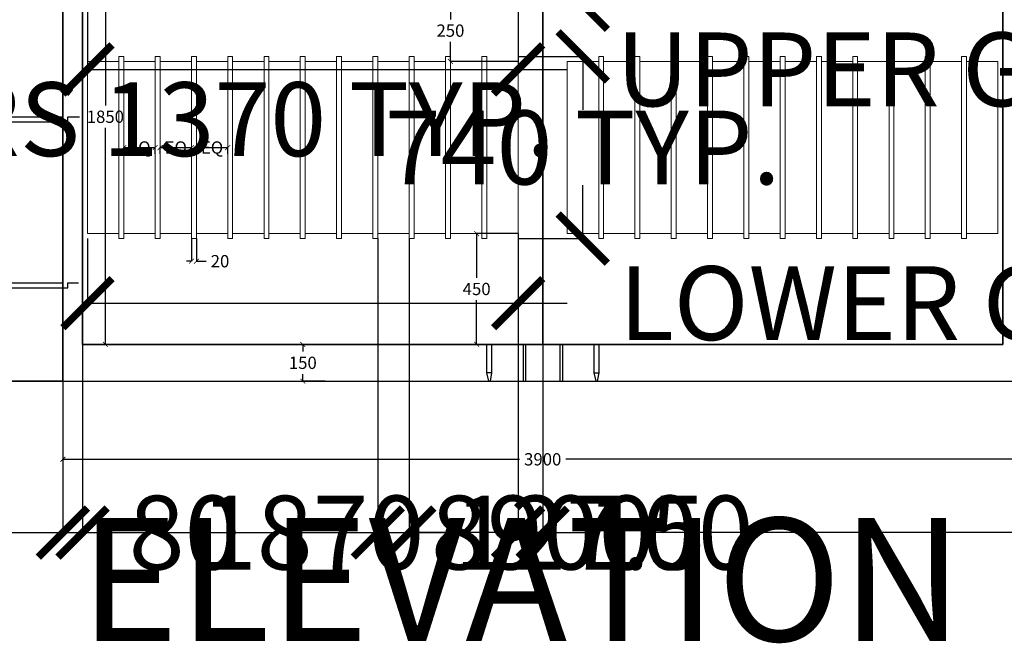
# Model space of a CAD drawing. Units: millimetres. Extents: x 16635 to 28332, y 17519 to 22633.
# Tile 2 of 4: x 20029 to 24031, y 17519 to 20054. Entities that reach past the tile are written whole.
import ezdxf
from ezdxf import colors
from ezdxf.entities.mleader import LeaderData, LeaderLine
from ezdxf.math import Vec2, Vec3

# ---------------------------------------------------------------- set-up
doc = ezdxf.new("R2010")
doc.units = ezdxf.units.MM
doc.header["$MEASUREMENT"] = 0
for name, color, linetype, lineweight in [('A-ANNO-DIMS', 2, 'Continuous', 18), ('A-ANNO-TEXT', 7, 'Continuous', 18), ('A-ELEV-GRAD', 7, 'Continuous', 30), ('A-GATE', 3, 'Continuous', 35), ('A-GATE-GRIL', 4, 'Continuous', 18), ('A-GATE-HRDW', 3, 'Continuous', 25), ('A-WALL', 7, 'Continuous', 35)]:
    doc.layers.add(name, color=color, linetype=linetype, lineweight=lineweight)
doc.styles.get("Standard").update_dxf_attribs({"font": 'arial.ttf'})
doc.dimstyles.get("Standard").update_dxf_attribs({"dimtxt": 300, "dimasz": 200, "dimexe": 0.18, "dimexo": 0.0625, "dimgap": 0.09, "dimtad": 0, "dimtih": 1, "dimtoh": 1, "dimdec": 0, "dimzin": 0, "dimdsep": 46, "dimtxsty": 'Standard', "dimblk": 'ARCHTICK', "dimcen": 0.09, "dimadec": 0, "dimazin": 0, "dimtfac": 1, "dimtdec": 0, "dimtofl": 0, "dimtmove": 0, "dimatfit": 3, "dimfxl": 1, "dimtolj": 1, "dimtzin": 0, "dimarcsym": 0})

# ---------------------------------------------------------------- blocks, each defined once
blk = doc.blocks.new('_ArchTick')
at = {"color": 0, "linetype": 'ByBlock', "const_width": 0.15}
blk.add_lwpolyline([(-0.5, -0.5), (0.5, 0.5)], dxfattribs=at)
blk = doc.blocks.new('*D13')
at = {"layer": 'A-ANNO-DIMS', "color": 0, "lineweight": -2, "transparency": 16777216}
for p, q in [((20284.8, 20584.3), (20377.6, 20584.3)), ((20377.4, 20584.3), (20377.4, 19704.9)), ((20377.4, 18734.3), (20377.4, 19613.8)), ((20284.8, 18734.3), (20377.6, 18734.3))]:
    blk.add_line(p, q, dxfattribs=at)
at = {"layer": 'Defpoints', "color": 0, "transparency": 16777216}
for p in [(20284.8, 20584.3), (20284.8, 18734.3), (20377.4, 18734.3)]:
    blk.add_point(p, dxfattribs=at)
at = {"layer": 'A-ANNO-DIMS', "color": 0, "lineweight": -2, "transparency": 16777216, "xscale": 20, "yscale": 20, "zscale": 20}
for p, rotation in [((20377.4, 20584.3), 90), ((20377.4, 18734.3), 270)]:
    blk.add_blockref('_ArchTick', p, dxfattribs=dict(at, rotation=rotation))
at = {"layer": 'A-ANNO-DIMS', "color": 0, "transparency": 16777216, "insert": (20377.4, 19659.3), "char_height": 50, "attachment_point": 5}
blk.add_mtext('\\A1;1850', dxfattribs=at)
blk = doc.blocks.new('*D14')
at = {"layer": 'A-ANNO-DIMS', "color": 0, "lineweight": -2, "transparency": 16777216}
for p, q in [((22054.7, 20134.3), (21779.6, 20134.3)), ((21779.8, 20134.3), (21779.8, 20054.9)), ((21779.8, 19884.3), (21779.8, 19963.8)), ((22054.7, 19884.3), (21779.6, 19884.3))]:
    blk.add_line(p, q, dxfattribs=at)
at = {"layer": 'Defpoints', "color": 0, "transparency": 16777216}
for p in [(22054.8, 20134.3), (21779.8, 19884.3), (22054.8, 19884.3)]:
    blk.add_point(p, dxfattribs=at)
at = {"layer": 'A-ANNO-DIMS', "color": 0, "lineweight": -2, "transparency": 16777216, "xscale": 20, "yscale": 20, "zscale": 20}
for p, rotation in [((21779.8, 20134.3), 90), ((21779.8, 19884.3), 270)]:
    blk.add_blockref('_ArchTick', p, dxfattribs=dict(at, rotation=rotation))
at = {"layer": 'A-ANNO-DIMS', "color": 0, "transparency": 16777216, "insert": (21779.8, 20009.3), "char_height": 50, "attachment_point": 5}
blk.add_mtext('\\A1;250', dxfattribs=at)
blk = doc.blocks.new('*D16')
at = {"layer": 'A-ANNO-DIMS', "color": 0, "lineweight": -2, "transparency": 16777216}
for p, q in [((21271.2, 18734.3), (21179.6, 18734.3)), ((21179.8, 18734.3), (21179.8, 18704.9)), ((21179.8, 18584.3), (21179.8, 18613.8)), ((21271.2, 18584.3), (21179.6, 18584.3))]:
    blk.add_line(p, q, dxfattribs=at)
at = {"layer": 'Defpoints', "color": 0, "transparency": 16777216}
for p in [(21179.8, 18734.3), (21271.2, 18734.3), (21271.2, 18584.3)]:
    blk.add_point(p, dxfattribs=at)
at = {"layer": 'A-ANNO-DIMS', "color": 0, "lineweight": -2, "transparency": 16777216, "xscale": 20, "yscale": 20, "zscale": 20}
for p, rotation in [((21179.8, 18734.3), 90), ((21179.8, 18584.3), 270)]:
    blk.add_blockref('_ArchTick', p, dxfattribs=dict(at, rotation=rotation))
at = {"layer": 'A-ANNO-DIMS', "color": 0, "transparency": 16777216, "insert": (21179.8, 18659.3), "char_height": 50, "attachment_point": 5}
blk.add_mtext('\\A1;150', dxfattribs=at)
blk = doc.blocks.new('*D17')
at = {"layer": 'A-ANNO-DIMS', "color": 0, "lineweight": -2, "transparency": 16777216}
for p, q in [((22054.7, 19184.3), (21886.1, 19184.3)), ((21886.3, 19184.3), (21886.3, 19004.9)), ((21886.3, 18734.3), (21886.3, 18913.8)), ((22054.7, 18734.3), (21886.1, 18734.3))]:
    blk.add_line(p, q, dxfattribs=at)
at = {"layer": 'Defpoints', "color": 0, "transparency": 16777216}
for p in [(22054.8, 19184.3), (21886.3, 18734.3), (22054.8, 18734.3)]:
    blk.add_point(p, dxfattribs=at)
at = {"layer": 'A-ANNO-DIMS', "color": 0, "lineweight": -2, "transparency": 16777216, "xscale": 20, "yscale": 20, "zscale": 20}
for p, rotation in [((21886.3, 19184.3), 90), ((21886.3, 18734.3), 270)]:
    blk.add_blockref('_ArchTick', p, dxfattribs=dict(at, rotation=rotation))
at = {"layer": 'A-ANNO-DIMS', "color": 0, "transparency": 16777216, "insert": (21886.3, 18959.3), "char_height": 50, "attachment_point": 5}
blk.add_mtext('\\A1;450', dxfattribs=at)
blk = doc.blocks.new('*D19')
at = {"layer": 'A-ANNO-DIMS', "color": 0, "lineweight": -2, "transparency": 16777216}
for p, q in [((20204.8, 18584.3), (20204.8, 18267)), ((24104.8, 18584.3), (24104.8, 18267)), ((20204.8, 18267.2), (22060.2, 18267.2)), ((24104.8, 18267.2), (22249.3, 18267.2))]:
    blk.add_line(p, q, dxfattribs=at)
at = {"layer": 'Defpoints', "color": 0, "transparency": 16777216}
for p in [(20204.8, 18584.3), (24104.8, 18584.3), (24104.8, 18267.2)]:
    blk.add_point(p, dxfattribs=at)
at = {"layer": 'A-ANNO-DIMS', "color": 0, "lineweight": -2, "transparency": 16777216, "xscale": 20, "yscale": 20, "zscale": 20, "rotation": 180}
blk.add_blockref('_ArchTick', (20204.8, 18267.2), dxfattribs=at)
at = {"layer": 'A-ANNO-DIMS', "color": 0, "lineweight": -2, "transparency": 16777216, "xscale": 20, "yscale": 20, "zscale": 20}
blk.add_blockref('_ArchTick', (24104.8, 18267.2), dxfattribs=at)
at = {"layer": 'A-ANNO-DIMS', "color": 0, "transparency": 16777216, "insert": (22154.8, 18267.2), "char_height": 50, "attachment_point": 5}
blk.add_mtext('\\A1;3900', dxfattribs=at)
blk = doc.blocks.new('*D28')
at = {"layer": 'A-ANNO-DIMS', "color": 0, "lineweight": -2, "transparency": 16777216}
for p, q in [((20727.3, 19164.3), (20727.3, 19072.1)), ((20747.3, 19164.3), (20747.3, 19072.1)), ((20727.3, 19072.3), (20707.3, 19072.3)), ((20747.3, 19072.3), (20787.3, 19072.3))]:
    blk.add_line(p, q, dxfattribs=at)
at = {"layer": 'Defpoints', "color": 0, "transparency": 16777216}
for p in [(20727.3, 19164.3), (20747.3, 19164.3), (20747.3, 19072.3)]:
    blk.add_point(p, dxfattribs=at)
at = {"layer": 'A-ANNO-DIMS', "color": 0, "lineweight": -2, "transparency": 16777216, "xscale": 20, "yscale": 20, "zscale": 20}
blk.add_blockref('_ArchTick', (20727.3, 19072.3), dxfattribs=at)
at = {"layer": 'A-ANNO-DIMS', "color": 0, "lineweight": -2, "transparency": 16777216, "xscale": 20, "yscale": 20, "zscale": 20, "rotation": 180}
blk.add_blockref('_ArchTick', (20747.3, 19072.3), dxfattribs=at)
at = {"layer": 'A-ANNO-DIMS', "color": 0, "transparency": 16777216, "insert": (20843.4, 19072.3), "char_height": 50, "attachment_point": 5}
blk.add_mtext('\\A1;20', dxfattribs=at)
blk = doc.blocks.new('*D32')
at = {"layer": 'A-ANNO-DIMS', "color": 0, "lineweight": -2, "transparency": 16777216}
for p, q in [((20452.3, 19508.7), (20452.3, 19534.5)), ((20452.3, 19534.3), (20579.8, 19534.3)), ((20579.8, 19508.7), (20579.8, 19534.5))]:
    blk.add_line(p, q, dxfattribs=at)
at = {"layer": 'Defpoints', "color": 0, "transparency": 16777216}
for p in [(20579.8, 19534.3), (20452.3, 19508.6), (20579.8, 19508.6)]:
    blk.add_point(p, dxfattribs=at)
at = {"layer": 'A-ANNO-DIMS', "color": 0, "lineweight": -2, "transparency": 16777216, "xscale": 20, "yscale": 20, "zscale": 20, "rotation": 180}
blk.add_blockref('_ArchTick', (20452.3, 19534.3), dxfattribs=at)
at = {"layer": 'A-ANNO-DIMS', "color": 0, "lineweight": -2, "transparency": 16777216, "xscale": 20, "yscale": 20, "zscale": 20}
blk.add_blockref('_ArchTick', (20579.8, 19534.3), dxfattribs=at)
at = {"layer": 'A-ANNO-DIMS', "color": 0, "transparency": 16777216, "insert": (20516, 19534.3), "char_height": 50, "attachment_point": 5}
blk.add_mtext('\\A1;EQ', dxfattribs=at)
blk = doc.blocks.new('*D33')
at = {"layer": 'A-ANNO-DIMS', "color": 0, "lineweight": -2, "transparency": 16777216}
for p, q in [((20599.8, 19508.7), (20599.8, 19534.5)), ((20599.8, 19534.3), (20727.3, 19534.3)), ((20727.3, 19508.7), (20727.3, 19534.5))]:
    blk.add_line(p, q, dxfattribs=at)
at = {"layer": 'Defpoints', "color": 0, "transparency": 16777216}
for p in [(20727.3, 19534.3), (20599.8, 19508.6), (20727.3, 19508.6)]:
    blk.add_point(p, dxfattribs=at)
at = {"layer": 'A-ANNO-DIMS', "color": 0, "lineweight": -2, "transparency": 16777216, "xscale": 20, "yscale": 20, "zscale": 20, "rotation": 180}
blk.add_blockref('_ArchTick', (20599.8, 19534.3), dxfattribs=at)
at = {"layer": 'A-ANNO-DIMS', "color": 0, "lineweight": -2, "transparency": 16777216, "xscale": 20, "yscale": 20, "zscale": 20}
blk.add_blockref('_ArchTick', (20727.3, 19534.3), dxfattribs=at)
at = {"layer": 'A-ANNO-DIMS', "color": 0, "transparency": 16777216, "insert": (20663.5, 19534.3), "char_height": 50, "attachment_point": 5}
blk.add_mtext('\\A1;EQ', dxfattribs=at)
blk = doc.blocks.new('*D34')
at = {"layer": 'A-ANNO-DIMS', "color": 0, "lineweight": -2, "transparency": 16777216}
for p, q in [((20747.3, 19508.7), (20747.3, 19534.5)), ((20747.3, 19534.3), (20874.8, 19534.3)), ((20874.8, 19508.7), (20874.8, 19534.5))]:
    blk.add_line(p, q, dxfattribs=at)
at = {"layer": 'Defpoints', "color": 0, "transparency": 16777216}
for p in [(20874.8, 19534.3), (20747.3, 19508.6), (20874.8, 19508.6)]:
    blk.add_point(p, dxfattribs=at)
at = {"layer": 'A-ANNO-DIMS', "color": 0, "lineweight": -2, "transparency": 16777216, "xscale": 20, "yscale": 20, "zscale": 20, "rotation": 180}
blk.add_blockref('_ArchTick', (20747.3, 19534.3), dxfattribs=at)
at = {"layer": 'A-ANNO-DIMS', "color": 0, "lineweight": -2, "transparency": 16777216, "xscale": 20, "yscale": 20, "zscale": 20}
blk.add_blockref('_ArchTick', (20874.8, 19534.3), dxfattribs=at)
at = {"layer": 'A-ANNO-DIMS', "color": 0, "transparency": 16777216, "insert": (20811, 19534.3), "char_height": 50, "attachment_point": 5}
blk.add_mtext('\\A1;EQ', dxfattribs=at)
blk = doc.blocks.new('GATE-GRILLE-LOWER')
for p, q in [((127.5, 720), (127.5, 740)), ((127.5, 740), (147.5, 740)), ((147.5, 740), (147.5, 720)), ((275, 720), (275, 740)), ((275, 740), (295, 740)), ((295, 740), (295, 720)), ((422.5, 720), (422.5, 740)), ((422.5, 740), (442.5, 740)), ((442.5, 740), (442.5, 720)), ((570, 720), (570, 740)), ((570, 740), (590, 740)), ((590, 740), (590, 720)), ((717.5, 720), (717.5, 740)), ((717.5, 740), (737.5, 740)), ((737.5, 740), (737.5, 720)), ((865, 720), (865, 740)), ((865, 740), (885, 740)), ((885, 740), (885, 720)), ((1012.5, 720), (1012.5, 740)), ((1012.5, 740), (1032.5, 740)), ((1032.5, 740), (1032.5, 720)), ((1160, 720), (1160, 740)), ((1160, 740), (1180, 740)), ((1180, 740), (1180, 720)), ((1307.5, 720), (1307.5, 740)), ((1307.5, 740), (1327.5, 740)), ((1327.5, 740), (1327.5, 720)), ((1455, 720), (1455, 740)), ((1455, 740), (1475, 740)), ((1475, 740), (1475, 720)), ((1602.5, 720), (1602.5, 740)), ((1602.5, 740), (1622.5, 740)), ((1622.5, 740), (1622.5, 720)), ((0, 720), (127.5, 720)), ((0, 720), (0, 20)), ((127.5, 720), (127.5, 20)), ((147.5, 720), (147.5, 20)), ((147.5, 720), (275, 720)), ((275, 720), (275, 20)), ((295, 720), (295, 20)), ((295, 720), (422.5, 720)), ((422.5, 720), (422.5, 20)), ((442.5, 720), (442.5, 20)), ((442.5, 720), (570, 720)), ((570, 720), (570, 20)), ((590, 720), (590, 20)), ((590, 720), (717.5, 720)), ((717.5, 720), (717.5, 20)), ((737.5, 720), (737.5, 20)), ((737.5, 720), (865, 720)), ((865, 720), (865, 20)), ((885, 720), (885, 20)), ((885, 720), (1012.5, 720)), ((1012.5, 720), (1012.5, 20)), ((1032.5, 720), (1032.5, 20)), ((1032.5, 720), (1160, 720)), ((1160, 720), (1160, 20)), ((1180, 720), (1180, 20)), ((1180, 720), (1307.5, 720)), ((1307.5, 720), (1307.5, 20)), ((1327.5, 720), (1327.5, 20)), ((1327.5, 720), (1455, 720)), ((1455, 720), (1455, 20)), ((1475, 720), (1475, 20)), ((1475, 720), (1602.5, 720)), ((1602.5, 720), (1602.5, 20)), ((1622.5, 720), (1622.5, 20)), ((1622.5, 720), (1750, 720)), ((1750, 720), (1750, 20)), ((0, 20), (127.5, 20)), ((127.5, 20), (127.5, 0)), ((147.5, 0), (147.5, 20)), ((147.5, 20), (275, 20)), ((275, 20), (275, 0)), ((295, 0), (295, 20)), ((295, 20), (422.5, 20)), ((422.5, 20), (422.5, 0)), ((442.5, 0), (442.5, 20)), ((442.5, 20), (570, 20)), ((570, 20), (570, 0)), ((590, 0), (590, 20)), ((590, 20), (717.5, 20)), ((717.5, 20), (717.5, 0)), ((737.5, 0), (737.5, 20)), ((737.5, 20), (865, 20)), ((865, 20), (865, 0)), ((885, 0), (885, 20)), ((885, 20), (1012.5, 20)), ((1012.5, 20), (1012.5, 0)), ((1032.5, 0), (1032.5, 20)), ((1032.5, 20), (1160, 20)), ((1160, 20), (1160, 0)), ((1180, 0), (1180, 20)), ((1180, 20), (1307.5, 20)), ((1307.5, 20), (1307.5, 0)), ((1327.5, 0), (1327.5, 20)), ((1327.5, 20), (1455, 20)), ((1455, 20), (1455, 0)), ((1475, 0), (1475, 20)), ((1475, 20), (1602.5, 20)), ((1602.5, 20), (1602.5, 0)), ((1622.5, 0), (1622.5, 20)), ((1622.5, 20), (1750, 20)), ((127.5, 0), (147.5, 0)), ((275, 0), (295, 0)), ((422.5, 0), (442.5, 0)), ((570, 0), (590, 0)), ((717.5, 0), (737.5, 0)), ((865, 0), (885, 0)), ((1012.5, 0), (1032.5, 0)), ((1160, 0), (1180, 0)), ((1307.5, 0), (1327.5, 0)), ((1455, 0), (1475, 0)), ((1602.5, 0), (1622.5, 0))]:
    blk.add_line(p, q)
blk = doc.blocks.new('GATE-JAMB-ANCHOR-SET')
for p, q in [((0.2, 1370), (297.2, 1370)), ((317.2, 1350), (317.2, 1370)), ((317.2, 1370), (351.9, 1370)), ((0.2, 1350), (297.2, 1350)), ((297.2, 1350), (317.2, 1350)), ((0, 694.8), (297, 694.8)), ((317, 674.8), (317, 694.8)), ((317, 694.8), (365.3, 694.8)), ((0, 674.8), (297, 674.8)), ((297, 674.8), (317, 674.8)), ((0.2, 20), (297.2, 20)), ((317.2, 0), (317.2, 20)), ((317.2, 20), (360.9, 20)), ((0.2, 0), (297.2, 0)), ((297.2, 0), (317.2, 0))]:
    blk.add_line(p, q)
blk = doc.blocks.new('*D43')
at = {"layer": 'A-ANNO-DIMS', "color": 0, "lineweight": -2, "transparency": 16777216}
for p, q in [((20304.8, 19164.3), (20304.8, 18901.7)), ((22054.8, 19164.3), (22054.8, 18901.7)), ((20304.8, 18901.8), (22054.8, 18901.8)), ((22054.8, 18901.8), (22254.8, 18901.8))]:
    blk.add_line(p, q, dxfattribs=at)
at = {"layer": 'Defpoints', "color": 0, "transparency": 16777216}
for p in [(20304.8, 19164.3), (22054.8, 19164.3), (22054.8, 18901.8)]:
    blk.add_point(p, dxfattribs=at)
at = {"layer": 'A-ANNO-DIMS', "color": 0, "lineweight": -2, "transparency": 16777216, "xscale": 200, "yscale": 200, "zscale": 200, "rotation": 180}
blk.add_blockref('_ArchTick', (20304.8, 18901.8), dxfattribs=at)
at = {"layer": 'A-ANNO-DIMS', "color": 0, "lineweight": -2, "transparency": 16777216, "xscale": 200, "yscale": 200, "zscale": 200}
blk.add_blockref('_ArchTick', (22054.8, 18901.8), dxfattribs=at)
at = {"layer": 'A-ANNO-DIMS', "color": 0, "transparency": 16777216, "insert": (24841.7, 18901.8), "char_height": 300, "attachment_point": 5}
blk.add_mtext('\\A1;LOWER GRILLE 1750 TYP.', dxfattribs=at)
blk = doc.blocks.new('*D44')
at = {"layer": 'A-ANNO-DIMS', "color": 0, "lineweight": -2, "transparency": 16777216}
for p, q in [((22054.8, 19904.3), (22317.5, 19904.3)), ((22317.3, 19904.3), (22317.3, 19687.6)), ((22317.3, 19164.3), (22317.3, 19381.1)), ((22054.8, 19164.3), (22317.5, 19164.3))]:
    blk.add_line(p, q, dxfattribs=at)
at = {"layer": 'Defpoints', "color": 0, "transparency": 16777216}
for p in [(22054.8, 19904.3), (22317.3, 19904.3), (22054.8, 19164.3)]:
    blk.add_point(p, dxfattribs=at)
at = {"layer": 'A-ANNO-DIMS', "color": 0, "lineweight": -2, "transparency": 16777216, "xscale": 200, "yscale": 200, "zscale": 200}
for p, rotation in [((22317.3, 19904.3), 90), ((22317.3, 19164.3), 270)]:
    blk.add_blockref('_ArchTick', p, dxfattribs=dict(at, rotation=rotation))
at = {"layer": 'A-ANNO-DIMS', "color": 0, "transparency": 16777216, "insert": (22317.3, 19534.3), "char_height": 300, "attachment_point": 5}
blk.add_mtext('\\A1;740 TYP.', dxfattribs=at)
blk = doc.blocks.new('*D45')
at = {"layer": 'A-ANNO-DIMS', "color": 0, "lineweight": -2, "transparency": 16777216}
for p, q in [((20304.8, 20114.3), (20304.8, 19851.7)), ((22054.8, 20114.3), (22054.8, 19851.7)), ((20304.8, 19851.8), (22054.8, 19851.8)), ((22054.8, 19851.8), (22254.8, 19851.8))]:
    blk.add_line(p, q, dxfattribs=at)
at = {"layer": 'Defpoints', "color": 0, "transparency": 16777216}
for p in [(20304.8, 20114.3), (22054.8, 20114.3), (22054.8, 19851.8)]:
    blk.add_point(p, dxfattribs=at)
at = {"layer": 'A-ANNO-DIMS', "color": 0, "lineweight": -2, "transparency": 16777216, "xscale": 200, "yscale": 200, "zscale": 200, "rotation": 180}
blk.add_blockref('_ArchTick', (20304.8, 19851.8), dxfattribs=at)
at = {"layer": 'A-ANNO-DIMS', "color": 0, "lineweight": -2, "transparency": 16777216, "xscale": 200, "yscale": 200, "zscale": 200}
blk.add_blockref('_ArchTick', (22054.8, 19851.8), dxfattribs=at)
at = {"layer": 'A-ANNO-DIMS', "color": 0, "transparency": 16777216, "insert": (24794.1, 19851.8), "char_height": 300, "attachment_point": 5}
blk.add_mtext('\\A1;UPPER GRILLE 1750 TYP.', dxfattribs=at)
blk = doc.blocks.new('*D46')
at = {"layer": 'A-ANNO-DIMS', "color": 0, "lineweight": -2, "transparency": 16777216}
for p, q in [((22054.8, 20525.3), (22317.5, 20525.3)), ((22317.3, 20525.3), (22317.3, 20470.7)), ((22317.3, 20114.3), (22317.3, 20169)), ((22054.8, 20114.3), (22317.5, 20114.3))]:
    blk.add_line(p, q, dxfattribs=at)
at = {"layer": 'Defpoints', "color": 0, "transparency": 16777216}
for p in [(22054.8, 20525.3), (22317.3, 20525.3), (22054.8, 20114.3)]:
    blk.add_point(p, dxfattribs=at)
at = {"layer": 'A-ANNO-DIMS', "color": 0, "lineweight": -2, "transparency": 16777216, "xscale": 200, "yscale": 200, "zscale": 200}
for p, rotation in [((22317.3, 20525.3), 90), ((22317.3, 20114.3), 270)]:
    blk.add_blockref('_ArchTick', p, dxfattribs=dict(at, rotation=rotation))
at = {"layer": 'A-ANNO-DIMS', "color": 0, "transparency": 16777216, "insert": (22317.3, 20319.8), "char_height": 300, "attachment_point": 5}
blk.add_mtext('\\A1;411 TYP.', dxfattribs=at)
blk = doc.blocks.new('*D47')
at = {"layer": 'A-ANNO-DIMS', "color": 0, "lineweight": -2, "transparency": 16777216}
for p, q in [((21092.8, 21187.8), (20990.3, 21187.8)), ((20990.5, 21187.8), (20990.5, 21001.9)), ((20990.5, 20505.3), (20990.5, 20691.3)), ((21092.8, 20505.3), (20990.3, 20505.3))]:
    blk.add_line(p, q, dxfattribs=at)
at = {"layer": 'Defpoints', "color": 0, "transparency": 16777216}
for p in [(20990.5, 21187.8), (21092.8, 21187.8), (21092.8, 20505.3)]:
    blk.add_point(p, dxfattribs=at)
at = {"layer": 'A-ANNO-DIMS', "color": 0, "lineweight": -2, "transparency": 16777216, "xscale": 200, "yscale": 200, "zscale": 200}
for p, rotation in [((20990.5, 21187.8), 90), ((20990.5, 20505.3), 270)]:
    blk.add_blockref('_ArchTick', p, dxfattribs=dict(at, rotation=rotation))
at = {"layer": 'A-ANNO-DIMS', "color": 0, "transparency": 16777216, "insert": (20990.5, 20846.6), "char_height": 300, "attachment_point": 5}
blk.add_mtext('\\A1;CREST SCROLL 682 TYP.', dxfattribs=at)
blk = doc.blocks.new('*D49')
at = {"layer": 'A-ANNO-DIMS', "color": 0, "lineweight": -2, "transparency": 16777216}
for p, q in [((19907.5, 20334.3), (19701.9, 20334.3)), ((19702.1, 20334.3), (19702.1, 19804.8)), ((19702.1, 18964.3), (19702.1, 19493.9)), ((19907.5, 18964.3), (19701.9, 18964.3))]:
    blk.add_line(p, q, dxfattribs=at)
at = {"layer": 'Defpoints', "color": 0, "transparency": 16777216}
for p in [(19702.1, 20334.3), (19907.6, 20334.3), (19907.6, 18964.3)]:
    blk.add_point(p, dxfattribs=at)
at = {"layer": 'A-ANNO-DIMS', "color": 0, "lineweight": -2, "transparency": 16777216, "xscale": 200, "yscale": 200, "zscale": 200}
for p, rotation in [((19702.1, 20334.3), 90), ((19702.1, 18964.3), 270)]:
    blk.add_blockref('_ArchTick', p, dxfattribs=dict(at, rotation=rotation))
at = {"layer": 'A-ANNO-DIMS', "color": 0, "transparency": 16777216, "insert": (19702.1, 19649.3), "char_height": 300, "attachment_point": 5}
blk.add_mtext('\\A1;JAMB ANCHORS 1370 TYP.', dxfattribs=at)
blk = doc.blocks.new('*D51')
at = {"layer": 'A-ANNO-DIMS', "color": 0, "lineweight": -2, "transparency": 16777216}
for p, q in [((17704.8, 18584.3), (17704.8, 17969.2)), ((26604.8, 18584.3), (26604.8, 17969.2)), ((17704.8, 17969.3), (21707, 17969.3)), ((26604.8, 17969.3), (22602.5, 17969.3))]:
    blk.add_line(p, q, dxfattribs=at)
at = {"layer": 'Defpoints', "color": 0, "transparency": 16777216}
for p in [(17704.8, 18584.3), (26604.8, 18584.3), (26604.8, 17969.3)]:
    blk.add_point(p, dxfattribs=at)
at = {"layer": 'A-ANNO-DIMS', "color": 0, "lineweight": -2, "transparency": 16777216, "xscale": 200, "yscale": 200, "zscale": 200, "rotation": 180}
blk.add_blockref('_ArchTick', (17704.8, 17969.3), dxfattribs=at)
at = {"layer": 'A-ANNO-DIMS', "color": 0, "lineweight": -2, "transparency": 16777216, "xscale": 200, "yscale": 200, "zscale": 200}
blk.add_blockref('_ArchTick', (26604.8, 17969.3), dxfattribs=at)
at = {"layer": 'A-ANNO-DIMS', "color": 0, "transparency": 16777216, "insert": (22154.8, 17969.3), "char_height": 300, "attachment_point": 5}
blk.add_mtext('\\A1;8900', dxfattribs=at)
blk = doc.blocks.new('*D55')
at = {"layer": 'A-ANNO-DIMS', "color": 0, "lineweight": -2, "transparency": 16777216}
for p, q in [((20284.8, 18734.3), (20284.8, 17969.2)), ((20204.8, 18584.3), (20204.8, 17969.2)), ((20204.8, 17969.3), (20284.8, 17969.3)), ((20284.8, 17969.3), (20484.8, 17969.3))]:
    blk.add_line(p, q, dxfattribs=at)
at = {"layer": 'Defpoints', "color": 0, "transparency": 16777216}
for p in [(20284.8, 18734.3), (20204.8, 18584.3), (20284.8, 17969.3)]:
    blk.add_point(p, dxfattribs=at)
at = {"layer": 'A-ANNO-DIMS', "color": 0, "lineweight": -2, "transparency": 16777216, "xscale": 200, "yscale": 200, "zscale": 200, "rotation": 180}
blk.add_blockref('_ArchTick', (20204.8, 17969.3), dxfattribs=at)
at = {"layer": 'A-ANNO-DIMS', "color": 0, "lineweight": -2, "transparency": 16777216, "xscale": 200, "yscale": 200, "zscale": 200}
blk.add_blockref('_ArchTick', (20284.8, 17969.3), dxfattribs=at)
at = {"layer": 'A-ANNO-DIMS', "color": 0, "transparency": 16777216, "insert": (20699.4, 17969.3), "char_height": 300, "attachment_point": 5}
blk.add_mtext('\\A1;80', dxfattribs=at)
blk = doc.blocks.new('*D56')
at = {"layer": 'A-ANNO-DIMS', "color": 0, "lineweight": -2, "transparency": 16777216}
for p, q in [((20284.8, 18734.3), (20284.8, 17969.2)), ((22154.8, 18734.3), (22154.8, 17969.2)), ((20284.8, 17969.3), (20786.4, 17969.3)), ((22154.8, 17969.3), (21653.2, 17969.3))]:
    blk.add_line(p, q, dxfattribs=at)
at = {"layer": 'Defpoints', "color": 0, "transparency": 16777216}
for p in [(20284.8, 18734.3), (22154.8, 18734.3), (22154.8, 17969.3)]:
    blk.add_point(p, dxfattribs=at)
at = {"layer": 'A-ANNO-DIMS', "color": 0, "lineweight": -2, "transparency": 16777216, "xscale": 200, "yscale": 200, "zscale": 200, "rotation": 180}
blk.add_blockref('_ArchTick', (20284.8, 17969.3), dxfattribs=at)
at = {"layer": 'A-ANNO-DIMS', "color": 0, "lineweight": -2, "transparency": 16777216, "xscale": 200, "yscale": 200, "zscale": 200}
blk.add_blockref('_ArchTick', (22154.8, 17969.3), dxfattribs=at)
at = {"layer": 'A-ANNO-DIMS', "color": 0, "transparency": 16777216, "insert": (21219.8, 17969.3), "char_height": 300, "attachment_point": 5}
blk.add_mtext('\\A1;1870', dxfattribs=at)
blk = doc.blocks.new('*D60')
at = {"layer": 'A-ANNO-DIMS', "color": 0, "lineweight": -2, "transparency": 16777216}
for p, q in [((22054.8, 19184.3), (22054.8, 17969.2)), ((22154.8, 18734.3), (22154.8, 17969.2)), ((22054.8, 17969.3), (22154.8, 17969.3)), ((22154.8, 17969.3), (22354.8, 17969.3))]:
    blk.add_line(p, q, dxfattribs=at)
at = {"layer": 'Defpoints', "color": 0, "transparency": 16777216}
for p in [(22054.8, 19184.3), (22154.8, 18734.3), (22154.8, 17969.3)]:
    blk.add_point(p, dxfattribs=at)
at = {"layer": 'A-ANNO-DIMS', "color": 0, "lineweight": -2, "transparency": 16777216, "xscale": 200, "yscale": 200, "zscale": 200, "rotation": 180}
blk.add_blockref('_ArchTick', (22054.8, 17969.3), dxfattribs=at)
at = {"layer": 'A-ANNO-DIMS', "color": 0, "lineweight": -2, "transparency": 16777216, "xscale": 200, "yscale": 200, "zscale": 200}
blk.add_blockref('_ArchTick', (22154.8, 17969.3), dxfattribs=at)
at = {"layer": 'A-ANNO-DIMS', "color": 0, "transparency": 16777216, "insert": (22671.6, 17969.3), "char_height": 300, "attachment_point": 5}
blk.add_mtext('\\A1;100', dxfattribs=at)
blk = doc.blocks.new('*D61')
at = {"layer": 'A-ANNO-DIMS', "color": 0, "lineweight": -2, "transparency": 16777216}
for p, q in [((21484.8, 19164.3), (21484.8, 17969.2)), ((21612.3, 19164.3), (21612.3, 17969.2)), ((21484.8, 17969.3), (21612.3, 17969.3)), ((21612.3, 17969.3), (21812.3, 17969.3))]:
    blk.add_line(p, q, dxfattribs=at)
at = {"layer": 'Defpoints', "color": 0, "transparency": 16777216}
for p in [(21484.8, 19164.3), (21612.3, 19164.3), (21612.3, 17969.3)]:
    blk.add_point(p, dxfattribs=at)
at = {"layer": 'A-ANNO-DIMS', "color": 0, "lineweight": -2, "transparency": 16777216, "xscale": 200, "yscale": 200, "zscale": 200, "rotation": 180}
blk.add_blockref('_ArchTick', (21484.8, 17969.3), dxfattribs=at)
at = {"layer": 'A-ANNO-DIMS', "color": 0, "lineweight": -2, "transparency": 16777216, "xscale": 200, "yscale": 200, "zscale": 200}
blk.add_blockref('_ArchTick', (21612.3, 17969.3), dxfattribs=at)
at = {"layer": 'A-ANNO-DIMS', "color": 0, "transparency": 16777216, "insert": (22305.5, 17969.3), "char_height": 300, "attachment_point": 5}
blk.add_mtext('\\A1;127.5', dxfattribs=at)

msp = doc.modelspace()

# ---------------------------------------------------------------- linework, layer by layer
at = {"layer": 'A-ELEV-GRAD'}
msp.add_line((20204.77, 18584.349), (24104.77, 18584.349), dxfattribs=at)
at = {"layer": 'A-GATE'}
for p, q in [((20284.77, 18734.349), (20284.77, 20585.349)), ((22154.77, 18734.349), (22154.77, 20585.349)), ((24024.77, 18734.349), (24024.77, 20585.349)), ((20284.77, 18734.349), (24024.77, 18734.349))]:
    msp.add_line(p, q, dxfattribs=at)
at = {"layer": 'A-GATE-HRDW'}
for p, q in [((21926.77, 18734.349), (21926.77, 18618.344)), ((21946.77, 18734.349), (21946.77, 18618.344)), ((22074.77, 18734.349), (22074.77, 18584.349)), ((22084.77, 18734.349), (22084.77, 18584.349)), ((22154.77, 18734.349), (22154.77, 18584.349)), ((22224.77, 18734.349), (22224.77, 18584.349)), ((22234.77, 18734.349), (22234.77, 18584.349)), ((22362.77, 18734.349), (22362.77, 18618.344)), ((22382.77, 18734.349), (22382.77, 18618.344)), ((21946.77, 18618.344), (21926.77, 18618.344)), ((21926.77, 18618.344), (21933.876, 18584.349)), ((21946.77, 18618.344), (21941.222, 18584.349)), ((22362.77, 18618.344), (22382.77, 18618.344)), ((22362.77, 18618.344), (22370.02, 18584.349)), ((22382.77, 18618.344), (22376.41, 18584.349))]:
    msp.add_line(p, q, dxfattribs=at)
at = {"layer": 'A-WALL'}
for p, q in [((20204.77, 18584.349), (20204.77, 21185.349)), ((18204.77, 18584.349), (20204.77, 18584.349))]:
    msp.add_line(p, q, dxfattribs=at)

# ---------------------------------------------------------------- block references
at = {"layer": 'A-GATE-GRIL'}
for p in [(20304.77, 19164.349), (22254.77, 19164.349)]:
    msp.add_blockref('GATE-GRILLE-LOWER', p, dxfattribs=at)
at = {"layer": 'A-GATE-HRDW'}
msp.add_blockref('GATE-JAMB-ANCHOR-SET', (19907.57, 18964.349), dxfattribs=at)

# ---------------------------------------------------------------- texts
at = {"layer": 'A-ANNO-TEXT'}
msp.add_text('ELEVATION', height=500, dxfattribs=at).set_placement((20273.527, 17528.228))

# ---------------------------------------------------------------- dimensions: what is measured, and where the dimension line sits
at = {"layer": 'A-ANNO-DIMS'}
for base, p1, p2, text, picture, middle in [((20990.466, 21187.833), (21092.839, 20505.349), (21092.839, 21187.833), 'CREST SCROLL <> TYP.', '*D47', (20990.466, 20846.591)), ((22317.27, 20525.349), (22054.77, 20114.349), (22054.77, 20525.349), '<> TYP.', '*D46', (22317.27, 20319.849)), ((19702.07, 20334.349), (19907.57, 18964.349), (19907.57, 20334.349), 'JAMB ANCHORS <> TYP.', '*D49', (19702.07, 19649.349)), ((22317.27, 19904.349), (22054.77, 19164.349), (22054.77, 19904.349), '<> TYP.', '*D44', (22317.27, 19534.349))]:
    dim = msp.add_linear_dim(base=base, p1=p1, p2=p2, angle=90, text=text, dimstyle='Standard', override={"dimdec": 0, "dimlfac": 1, "dimrnd": 0, "dimzin": 0, "dimdsep": 46, "dimlunit": 2}, dxfattribs=at)
    dim.commit()
    dim.dimension.update_dxf_attribs({"geometry": picture, "text_midpoint": middle})
for base, p1, p2, text, picture, middle in [((22054.77, 19851.849), (20304.77, 20114.349), (22054.77, 20114.349), 'UPPER GRILLE <> TYP.', '*D45', (24794.117, 19851.849)), ((22054.77, 18901.849), (20304.77, 19164.349), (22054.77, 19164.349), 'LOWER GRILLE <> TYP.', '*D43', (24841.695, 18901.849))]:
    dim = msp.add_linear_dim(base=base, p1=p1, p2=p2, text=text, dimstyle='Standard', override={"dimdec": 0, "dimlfac": 1, "dimrnd": 0, "dimzin": 0, "dimdsep": 46, "dimlunit": 2}, dxfattribs=at)
    dim.commit()
    dim.dimension.update_dxf_attribs({"geometry": picture, "text_midpoint": middle})
for base, p1, p2, picture, middle in [((20377.407, 18734.349), (20284.77, 20584.349), (20284.77, 18734.349), '*D13', (20377.407, 19659.349)), ((21886.328, 18734.349), (22054.77, 19184.349), (22054.77, 18734.349), '*D17', (21886.328, 18959.349))]:
    dim = msp.add_linear_dim(base=base, p1=p1, p2=p2, angle=90, dimstyle='Standard', override={"dimtxt": 50, "dimasz": 20, "dimgap": 20, "dimclrd": 0, "dimclre": 0, "dimclrt": 0}, dxfattribs=at)
    dim.commit()
    dim.dimension.update_dxf_attribs({"geometry": picture, "text_midpoint": middle, "dimtype": 160})
for base, p1, p2, picture, middle in [((21779.77, 19884.349), (22054.77, 20134.349), (22054.77, 19884.349), '*D14', (21779.77, 20009.349)), ((21179.773, 18734.349), (21271.245, 18584.349), (21271.245, 18734.349), '*D16', (21179.773, 18659.349))]:
    dim = msp.add_linear_dim(base=base, p1=p1, p2=p2, angle=90, dimstyle='Standard', override={"dimtxt": 50, "dimasz": 20, "dimgap": 20, "dimclrd": 0, "dimclre": 0, "dimclrt": 0}, dxfattribs=at)
    dim.commit()
    dim.dimension.update_dxf_attribs({"geometry": picture, "text_midpoint": middle})
for base, p1, p2, picture, middle in [((20579.77, 19534.299), (20452.27, 19508.611), (20579.77, 19508.611), '*D32', (20516.02, 19534.299)), ((20727.27, 19534.299), (20599.77, 19508.611), (20727.27, 19508.611), '*D33', (20663.52, 19534.299)), ((20874.77, 19534.299), (20747.27, 19508.611), (20874.77, 19508.611), '*D34', (20811.02, 19534.299))]:
    dim = msp.add_linear_dim(base=base, p1=p1, p2=p2, text='EQ', dimstyle='Standard', override={"dimtxt": 50, "dimasz": 20, "dimgap": 20, "dimclrd": 0, "dimclre": 0, "dimclrt": 0}, dxfattribs=at)
    dim.commit()
    dim.dimension.update_dxf_attribs({"geometry": picture, "text_midpoint": middle, "dimtype": 160})
for base, p1, p2, override, picture, middle in [((22154.77, 17969.349), (22054.77, 19184.349), (22154.77, 18734.349), {"dimdec": 0, "dimlfac": 1, "dimrnd": 0, "dimzin": 0, "dimdsep": 46, "dimlunit": 2}, '*D60', (22671.641, 17969.349)), ((20747.27, 19072.307), (20727.27, 19164.349), (20747.27, 19164.349), {"dimtxt": 50, "dimasz": 20, "dimgap": 20, "dimclrd": 0, "dimclre": 0, "dimclrt": 0}, '*D28', (20843.423, 19072.307)), ((21612.27, 17969.349), (21484.77, 19164.349), (21612.27, 19164.349), {"dimdec": 1, "dimlfac": 1, "dimrnd": 0, "dimzin": 0, "dimdsep": 46, "dimlunit": 2}, '*D61', (22305.539, 17969.349)), ((20284.77, 17969.349), (20204.77, 18584.349), (20284.77, 18734.349), {"dimdec": 0, "dimlfac": 1, "dimrnd": 0, "dimzin": 0, "dimdsep": 46, "dimlunit": 2}, '*D55', (20699.424, 17969.349)), ((22154.77, 17969.349), (20284.77, 18734.349), (22154.77, 18734.349), {"dimdec": 0, "dimlfac": 1, "dimrnd": 0, "dimzin": 0, "dimdsep": 46, "dimlunit": 2}, '*D56', (21219.77, 17969.349)), ((26604.77, 17969.349), (17704.77, 18584.349), (26604.77, 18584.349), {"dimdec": 0, "dimlfac": 1, "dimrnd": 0, "dimzin": 0, "dimdsep": 46, "dimlunit": 2}, '*D51', (22154.77, 17969.349)), ((24104.77, 18267.158), (20204.77, 18584.349), (24104.77, 18584.349), {"dimtxt": 50, "dimasz": 20, "dimgap": 20, "dimclrd": 0, "dimclre": 0, "dimclrt": 0}, '*D19', (22154.77, 18267.158))]:
    dim = msp.add_linear_dim(base=base, p1=p1, p2=p2, dimstyle='Standard', override=override, dxfattribs=at)
    dim.commit()
    dim.dimension.update_dxf_attribs({"geometry": picture, "text_midpoint": middle})

# ---------------------------------------------------------------- leaders
at = {"layer": 'A-ANNO-TEXT'}
ml = msp.add_multileader_mtext('Standard', dxfattribs=at)
ml.set_content('SAND\\\\STONE\\\\TIL\\PCLADDIND', color=256)
ml.set_leader_properties()
ml.build(insert=Vec2(0, 0))
ml.multileader.update_dxf_attribs({"dogleg_length": 0.36, "arrow_head_size": 120})
ctx = ml.context
ctx.base_point, ctx.char_height, ctx.arrow_head_size, ctx.landing_gap_size, ctx.plane_origin = Vec3(22967.113, 22389.231), 80, 120, 0.09, Vec3(23877.721, 22389.231)
ctx.text_align_type = 2
notes = []
notes.append((ctx, [(0, (1, 1, 0), (23877.721, 22389.231), (-1, 0), 0.36, [(0, [(24689.11, 19800.774), (24689.11, 22389.231)], 0, [])])]))
ctx.mtext.insert, ctx.mtext.alignment, ctx.mtext.flow_direction = Vec3(23877.271, 22429.914), 3, 5
for ctx, leaders in notes:
    for number, flags, end, landing, length, lines in leaders:
        leader = LeaderData()
        leader.index, (leader.has_last_leader_line, leader.has_dogleg_vector, leader.attachment_direction) = number, flags
        leader.last_leader_point, leader.dogleg_vector, leader.dogleg_length = Vec3(end), Vec3(landing), length
        for number, points, colour, breaks in lines:
            line = LeaderLine()
            line.index, line.vertices, line.color, line.breaks = number, Vec3.list(points), colors.encode_raw_color(colour), breaks
            leader.lines.append(line)
        ctx.leaders.append(leader)

doc.saveas('drawing.dxf')
